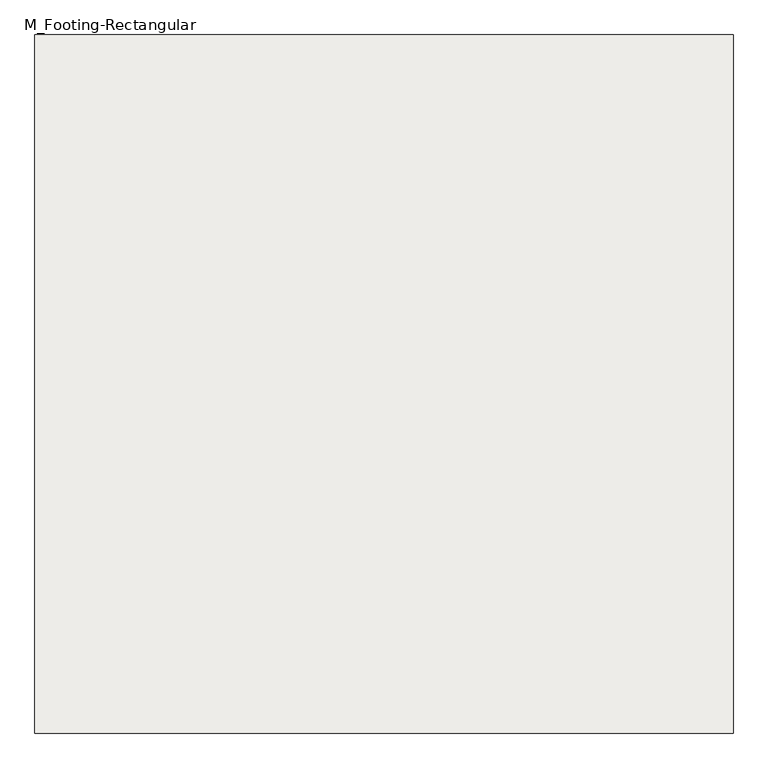
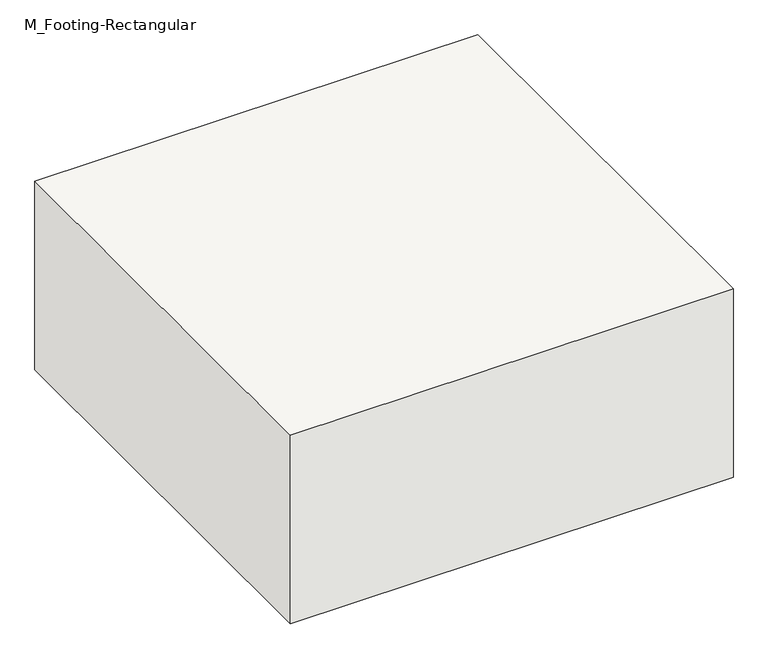
"""IFC4 building model written with IfcOpenShell, lengths in millimetres: slab geometry, M_Footing-Rectangular."""

from ifc_helpers import new_model, si_unit, frame, origin, place, context, project, spatial, polyline, outline, extrude, source, transform, mapped, element, save


def m_footing_rectangular_4c97ae35(model_context):
    return source(origin(), model_context, "Body", "SweptSolid", [
        extrude(outline(polyline([(500.0, 500.0), (500.0, -500.0), (-500.0, -500.0), (-500.0, 500.0), (500.0, 500.0)])), frame((0.0, 0.0, -450.0), z_axis=(0.0, 0.0, 1.0), x_axis=(1.0, 0.0, 0.0)), (0.0, 0.0, 1.0), 450.0),
    ])


if __name__ == "__main__":
    model = new_model("IFC4")
    model_context = context("Model", 3, world=origin())
    ifc_project = project(units=[si_unit("LENGTHUNIT", "METRE", prefix="MILLI")], contexts=[model_context])
    site = spatial("IfcSite", under=ifc_project)
    building = spatial("IfcBuilding", under=site)
    placement = place(None, origin())
    m_footing_rectangular_shape = m_footing_rectangular_4c97ae35(model_context)
    element("IfcSlab", 1, ObjectType="M_Footing-Rectangular", at=placement, inside=building, context=model_context, shape_type="MappedRepresentation", body=[
        mapped(m_footing_rectangular_shape, transform((0.0, 0.0, 0.0), x_axis=(1.0, 0.0, 0.0), y_axis=(0.0, 1.0, 0.0), z_axis=(0.0, 0.0, 1.0))),
    ])
    save(model, "model.ifc")

# Revit data of these elements
# Type "M_Footing-Rectangular"
#   Width = 1000 mm
#   Length = 1000 mm
#   Foundation Thickness = 450 mm
#   Structural Material [instance default] = Concrete, Cast-in-Place gray
#   Assembly Code = ""
# Element 1 (IfcSlab, "M_Footing-Rectangular")
#   Materials on its faces: "Concrete, Cast-in-Place gray"
# Materials
#   "Concrete, Cast-in-Place gray": class "Concrete", colour RGB 192 192 192, transparency 0, Description = "Cast-in-place concrete", Cost = 0
